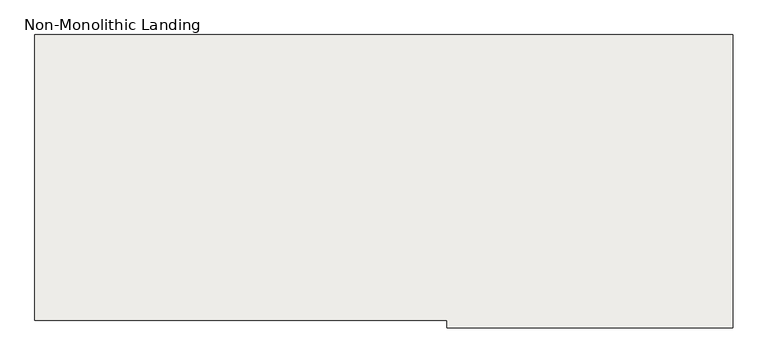
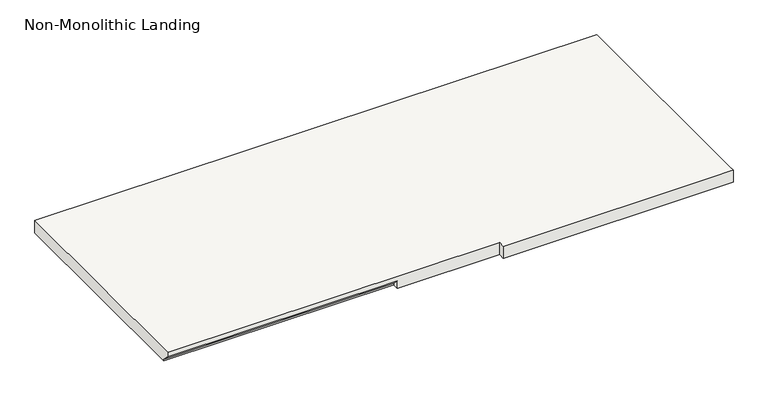
"""IFC4 building model written with IfcOpenShell, lengths in millimetres: slab geometry, Non-Monolithic Landing."""

from ifc_helpers import new_model, si_unit, origin, place, context, project, spatial, faceted_brep, source, transform, mapped, element, save


def non_monolithic_landing_71f31ac1(model_context):
    return source(origin(), model_context, "Body", "Brep", [
        faceted_brep([(-3617.4415084, -19522.1851539, 45874.2339133), (-3617.4415084, -19496.7851539, 45848.8339133), (-2703.0415084, -19496.7851539, 45848.8339133), (-2703.0415084, -19522.1851539, 45874.2339133), (-2296.6415084, -19522.1851539, 45893.2839133), (-2296.6415084, -19547.5851539, 45893.2839133), (-1382.2415084, -19547.5851539, 45893.2839133), (-1382.2415084, -19522.1851539, 45893.2839133), (-1382.2415084, -18607.7851539, 45893.2839133), (-3617.4415084, -18607.7851539, 45893.2839133), (-3617.4415084, -19522.1851539, 45893.2839133), (-2703.0415084, -19496.7851539, 45842.4839133), (-3617.4415084, -19496.7851539, 45842.4839133), (-3617.4415084, -18607.7851539, 45842.4839133), (-1382.2415084, -18607.7851539, 45842.4839133), (-1382.2415084, -19522.1851539, 45842.4839133), (-1382.2415084, -19547.5851539, 45842.4839133), (-2296.6415084, -19547.5851539, 45842.4839133), (-2296.6415084, -19522.1851539, 45842.4839133), (-2703.0415084, -19522.1851539, 45842.4839133)], [[[0, 1, 2, 3]], [[4, 5, 6, 7, 8, 9, 10]], [[11, 12, 13, 14, 15, 16, 17, 18, 19]], [[12, 11, 2, 1]], [[11, 19, 3, 2]], [[4, 10, 0, 3, 19, 18]], [[5, 4, 18, 17]], [[6, 5, 17, 16]], [[7, 6, 16, 15]], [[8, 7, 15, 14]], [[9, 8, 14, 13]], [[10, 9, 13, 12, 1, 0]]]),
    ])


if __name__ == "__main__":
    model = new_model("IFC4")
    model_context = context("Model", 3, world=origin())
    ifc_project = project(units=[si_unit("LENGTHUNIT", "METRE", prefix="MILLI")], contexts=[model_context])
    site = spatial("IfcSite", under=ifc_project)
    building = spatial("IfcBuilding", under=site)
    placement = place(None, origin())
    non_monolithic_landing_shape = non_monolithic_landing_71f31ac1(model_context)
    element("IfcSlab", 1, ObjectType="Non-Monolithic Landing", at=placement, inside=building, context=model_context, shape_type="MappedRepresentation", body=[
        mapped(non_monolithic_landing_shape, transform((0.0, 0.0, 0.0), x_axis=(1.0, 0.0, 0.0), y_axis=(0.0, 1.0, 0.0), z_axis=(0.0, 0.0, 1.0))),
    ])
    save(model, "model.ifc")
